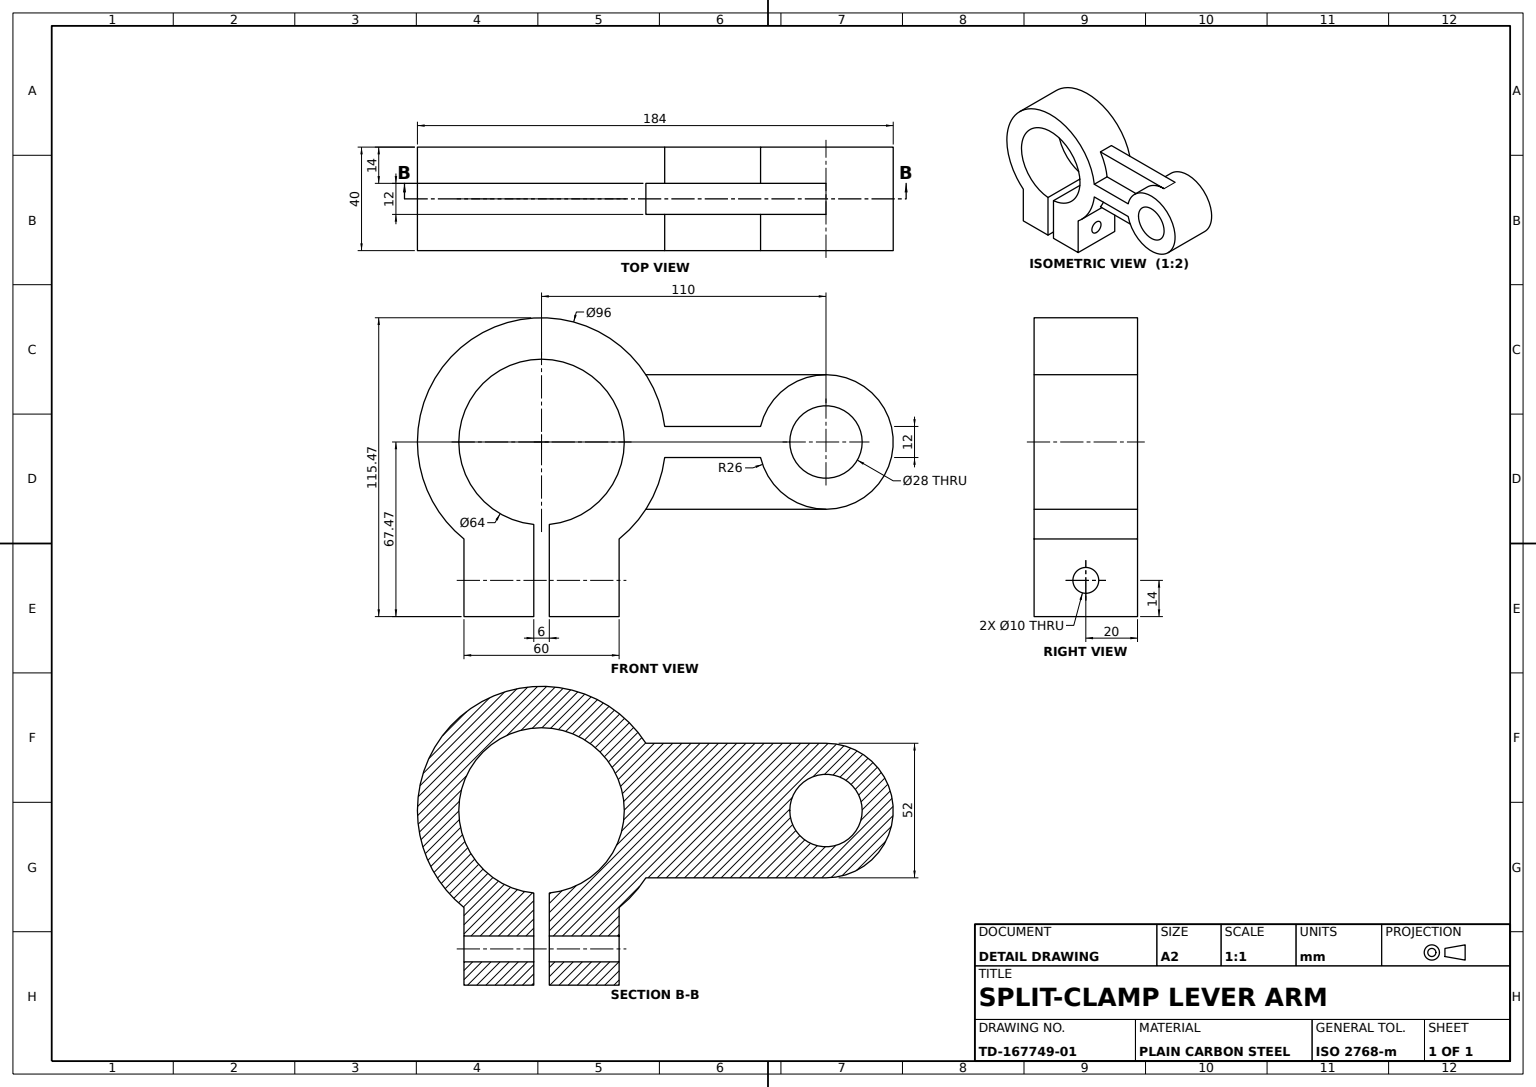
from build123d import *

# Parameters (mm, degrees)
CLAMP_RING_PROFILE_R       = 48
CLAMP_RING_96_DEPTH        = 20
END_BOSS_PROFILE_R         = 26
END_BOSS_52_DEPTH          = 20
LEVER_WEB_DEPTH            = 40
RIB_A_DEPTH                = 6
RIB_B_DEPTH                = 6
CLAMP_BORE_PROFILE_R       = 32
CLAMP_BORE_DEPTH           = 213
END_BORE_PROFILE_R         = 14
END_BORE_DEPTH             = 213
CLAMP_LUG_DEPTH            = 40
CLAMP_SLOT_DEPTH           = 40
CLAMP_SCREW_HOLE_PROFILE_R = 5
CLAMP_SCREW_HOLE_DEPTH     = 105


with BuildPart() as part:
    # Clamp Ring Profile → Clamp Ring Ø96 (new, symmetric)
    with BuildSketch(Plane.XY):
        Circle(CLAMP_RING_PROFILE_R)
    extrude(amount=CLAMP_RING_96_DEPTH, both=True)



with BuildPart() as body_2:
    # End Boss Profile → End Boss Ø52 (new, symmetric)
    with BuildSketch(Plane.XY):
        with Locations((110, 0)):
            Circle(END_BOSS_PROFILE_R)
    extrude(amount=END_BOSS_52_DEPTH, both=True)


with BuildPart() as part_1:
    add(part.part)

    add(body_2.part)  # Lever Web merges body 2
    # Lever Web Profile → Lever Web (add)
    with BuildSketch(Plane.XY.offset(20)):
        Polygon((48, 6), (86.790548166, 6), (86.790548166, -6), (44, -6), (44, 6), align=None)
    extrude(amount=-LEVER_WEB_DEPTH)

    # Rib A Profile → Rib A (add, symmetric)
    with BuildSketch(Plane.XY):
        with BuildLine():
            Line((110, 26), (40.348482004, 26))
            ThreePointArc((40.348482004, 26), (45.108407669, 16.408277105), (47.623523599, 6))
            Line((47.623523599, 6), (84.701778719, 6))
            ThreePointArc((84.701778719, 6), (93.875484503, 20.396078054), (110, 26))
        make_face()
    extrude(amount=RIB_A_DEPTH, both=True)

    # Rib B Profile → Rib B (add, symmetric)
    with BuildSketch(Plane.XY):
        with BuildLine():
            Line((110, -26), (40.276028999, -26))
            ThreePointArc((40.276028999, -26), (45.014976817, -16.391327753), (47.623523599, -6))
            Line((47.623523599, -6), (84.701778719, -6))
            ThreePointArc((84.701778719, -6), (93.875484503, -20.396078054), (110, -26))
        make_face()
    extrude(amount=RIB_B_DEPTH, both=True)

    # Clamp Bore Profile → Clamp Bore (cut)
    with BuildSketch(Plane.XY.offset(20)):
        Circle(CLAMP_BORE_PROFILE_R)
    extrude(amount=-CLAMP_BORE_DEPTH, mode=Mode.SUBTRACT)

    # End Bore Profile → End Bore (cut)
    with BuildSketch(Plane.XY.offset(20)):
        with Locations((110, 0)):
            Circle(END_BORE_PROFILE_R)
    extrude(amount=-END_BORE_DEPTH, mode=Mode.SUBTRACT)

    # Clamp Lug Profile → Clamp Lug (add)
    with BuildSketch(Plane.XY.offset(20)):
        Polygon((0, -37.46998799), (30, -37.46998799), (30, -67.46998799), (-30, -67.46998799), (-30, -37.46998799), align=None)
    extrude(amount=-CLAMP_LUG_DEPTH)

    # Clamp Slot Profile → Clamp Slot (cut)
    with BuildSketch(Plane.XY.offset(20)):
        Polygon((0, -67.46998799), (3, -67.46998799), (3, -25.366050336), (-3, -25.366050336), (-3, -67.46998799), align=None)
    extrude(amount=-CLAMP_SLOT_DEPTH, mode=Mode.SUBTRACT)

    # Clamp Screw Hole Profile → Clamp Screw Hole (cut)
    with BuildSketch(Plane(origin=(30, 0, 0), x_dir=(0, 0, -1), z_dir=(1, 0, 0))):
        with Locations(Location((0, -53.46998799, 0), (0, 0, 90))):
            Circle(CLAMP_SCREW_HOLE_PROFILE_R)
    extrude(amount=-CLAMP_SCREW_HOLE_DEPTH, mode=Mode.SUBTRACT)


solid = part_1.part
